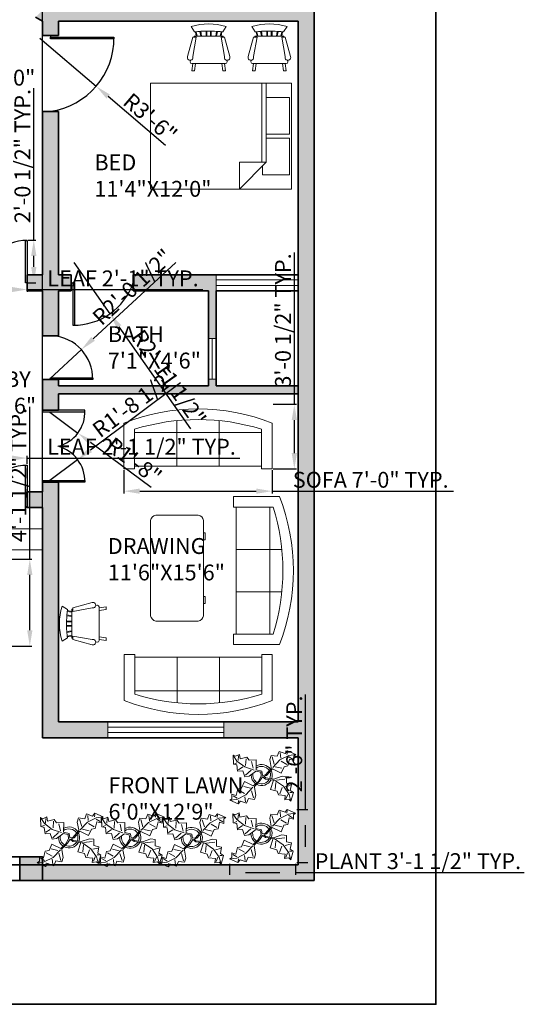
# Model space of a CAD drawing. Units: inches. Extents: x 32476 to 33108, y 58720 to 59630.
# Tile 5 of 6: x 32810 to 33096, y 58720 to 59278. Entities that reach past the tile are written whole.
import ezdxf

# ---------------------------------------------------------------- set-up
doc = ezdxf.new("R2010")
doc.units = ezdxf.units.IN
for name, color, linetype, lineweight in [('A-ANNO-DIMS', 6, 'Continuous', 18), ('A-ANNO-TTLB', 7, 'Continuous', 35), ('A-AREA-IDEN', 32, 'Continuous', 18), ('A-DOOR', 4, 'Continuous', 25), ('A-FLOR-STRS', 7, 'Continuous', 18), ('A-FURN', 8, 'Continuous', 18), ('A-GLAZ', 4, 'Continuous', 18), ('A-SITE-GATE', 7, 'Continuous', 35), ('A-SITE-PATT', 242, 'Continuous', 13), ('A-WALL', 7, 'Continuous', 35), ('A-WALL-PATT', 251, 'Continuous', 13), ('L-PLNT', 3, 'Continuous', 13)]:
    doc.layers.add(name, color=color, linetype=linetype, lineweight=lineweight)
doc.styles.get("Standard").update_dxf_attribs({"font": 'arial.ttf'})
doc.dimstyles.new('ISO-25', dxfattribs={"dimtxt": 9, "dimasz": 9, "dimexe": 1.25, "dimexo": 0.625, "dimtad": 1, "dimdec": 1, "dimrnd": 9, "dimlunit": 3, "dimtxsty": 'Standard', "dimcen": 2.5, "dimadec": 0, "dimazin": 0, "dimtfac": 1, "dimtdec": 1, "dimtmove": 0, "dimatfit": 3, "dimfxl": 1, "dimarcsym": 0})

# ---------------------------------------------------------------- blocks, each defined once
blk = doc.blocks.new('Bed - Queen')
for p, q in [((0, -80.00003), (0, 0)), ((0, 0), (59.99999, 0)), ((59.99999, 0), (59.99999, -80.00003)), ((7.99999, -1.2), (28.79998, -1.2)), ((7.99999, -14.4), (7.99999, -1.2)), ((28.79998, -1.2), (28.79998, -14.4)), ((31.19999, -1.2), (51.99999, -1.2)), ((31.19999, -14.4), (31.19999, -1.2)), ((51.99999, -1.2), (51.99999, -16.4)), ((0, -14.4), (44.8, -14.4)), ((59.99999, -29.6), (44.8, -14.4)), ((44.8, -14.4), (44.8, -29.6)), ((51.99999, -16.4), (46.79936, -16.4)), ((44.8, -16.8), (0, -16.8)), ((44.8, -29.6), (59.99999, -29.6)), ((59.99999, -80.00003), (0, -80.00003))]:
    blk.add_line(p, q)
blk = doc.blocks.new('Chair - Rocking')
for p, q in [((-8, -4.5), (-10, -1.5)), ((-7.5, -4.5), (-7, -7)), ((-6.5, -7), (-7.02225, -4.43)), ((-4.5, -7), (-4.96674, -4.19951)), ((-4, -7), (-4.40532, -4.16272)), ((-1.5, -4.05012), (-1.5, -7)), ((-1, -7), (-1, -4.05012)), ((1, -7), (1, -4.04655)), ((1.5, -4.05012), (1.5, -7)), ((4, -7), (4.40187, -4.18694)), ((4.5, -7), (4.96761, -4.19437)), ((6.5, -7), (7, -4.4057)), ((7.5, -4.5), (7, -7)), ((8, -4.5), (10, -1.5)), ((-9, -7.5), (-12, -18.49999)), ((-7, -7.5), (-9, -7.5)), ((-9, -18.49999), (-7, -7.5)), ((-8.23428, -6.99939), (-8.3093, -7.47958)), ((-8.23041, -7), (8.23915, -7)), ((7, -7.5), (9, -7.5)), ((9, -18.49999), (7, -7.5)), ((8.31071, -7.48854), (8.23449, -7.00073)), ((9, -7.5), (12, -18.49999)), ((-10.36644, -20.64523), (-10.5, -21.49999)), ((10.5, -21.49999), (10.3575, -20.58798)), ((-9, -22.49999), (-9.5, -26.49999)), ((0, -22.49999), (-9.5, -22.49999)), ((-9.5, -26.49999), (-8, -26.49999)), ((-8, -26.49999), (-7.5, -22.49999)), ((0, -22.49999), (9.5, -22.49999)), ((8, -26.49999), (7.5, -22.49999)), ((9.5, -26.49999), (8, -26.49999)), ((9, -22.49999), (9.5, -26.49999))]:
    blk.add_line(p, q)
for centre, radius, start, end in [((0, -34.08333), 34.08333, 72.93847, 107.0615), ((0, -68.25004), 64.25, 93.92211, 97.15267), ((0, -68.25004), 64.25, 82.84733, 93.92211), ((-10.5, -18.99999), 1.58114, 161.5651, 18.43495), ((-9.5, -21.49999), 1, 180, 270), ((10.5, -18.99999), 1.58114, 161.5651, 18.43495), ((9.5, -21.49999), 1, 270, 0)]:
    blk.add_arc(centre, radius, start, end)
blk = doc.blocks.new('Sofa - Roundback 7 ft.')
for p, q in [((-12.00002, -32.4421), (-12.00003, -6.5971)), ((11.99997, -32.4421), (11.99998, -6.5971)), ((-36.000027, -34), (-36.000027, -11.4696)), ((-35.999844, -13.3819), (35.9998, -13.3819)), ((35.99998, -34), (35.99998, -11.4696)), ((-36.000027, -32.4421), (35.99998, -32.4421))]:
    blk.add_line(p, q)
for points in [[(-36.000027, -34), (-42.000027, -34), (-42.000027, -8)], [(41.99998, -8), (41.99998, -34), (35.99998, -34)]]:
    blk.add_lwpolyline(points)
for centre, radius, start, end in [((0, -114.25), 114.25, 68.43141, 111.5686), ((-0.00001, -127.1968), 121.1968, 72.72033, 107.2797)]:
    blk.add_arc(centre, radius, start, end)
blk = doc.blocks.new('Desk - 30 x 60 in.')
for p, q in [((-26.999995, 0), (26.999995, 0)), ((-29.999995, -27), (-29.999995, -3)), ((29.999995, -3), (29.999995, -27)), ((26.999995, -30), (-26.999995, -30)), ((-20.000005, -30), (-20.000005, -31)), ((-20.000005, -31), (-16.000005, -31)), ((-16.000005, -31), (-16.000005, -30)), ((15.999995, -31), (15.999995, -30)), ((19.999995, -31), (15.999995, -31)), ((19.999995, -30), (19.999995, -31))]:
    blk.add_line(p, q)
for centre, start, end in [((-26.499995, -3.5), 98.1301, 171.8699), ((26.499995, -3.5), 8.130102, 81.8699), ((-26.499995, -26.5), 188.1301, 261.8699), ((26.499995, -26.5), 278.1301, 351.8699)]:
    blk.add_arc(centre, 3.535534, start, end)
blk = doc.blocks.new('Plant - Rubber or Philodendron')
for p, q in [((-16.2005, 11.4774), (-13.9899, 8.1064)), ((-16.2005, 11.4774), (-14.8639, 10.7964)), ((-16.0159, 6.3329), (-16.2005, 11.4774)), ((-14.8639, 10.7964), (-12.6195, 11.8975)), ((-12.6195, 11.8975), (-12.1909, 9.4345)), ((4.6914, 8.8812), (5.3859, 11.2828)), ((5.3859, 11.2828), (8.8871, 10.7908)), ((8.8871, 10.7908), (9.9809, 13.4933)), ((9.9809, 13.4933), (13.3837, 12.301)), ((15.3859, 11.3055), (10.3916, 8.7942)), ((10.5828, 12.6946), (10.8893, 9.7953)), ((13.3837, 12.301), (14.68, 13.9039)), ((14.5816, 13.2037), (14.3848, 11.8033)), ((14.68, 13.9039), (19.3848, 11.8146)), ((19.3848, 11.8146), (15.3859, 11.3055)), ((19.3848, 11.8146), (18.1868, 10.9119)), ((-14.0069, 5.8704), (-16.0159, 6.3329)), ((-15.3434, 6.5514), (-13.9984, 6.9884)), ((-13.5868, 2.2894), (-14.0069, 5.8704)), ((-13.9899, 8.1064), (-9.5434, 4.7185)), ((-13.3174, 8.325), (-13.0735, 11.0065)), ((-12.1909, 9.4345), (-8.3829, 10.3)), ((-8.8369, 9.409), (-9.0894, 5.6095)), ((-8.3829, 10.3), (-7.0549, 8.501)), ((-7.0549, 8.501), (-3.0284, 8.6941)), ((-4.8529, 4.012), (-5.7184, 7.82)), ((-3.0284, 8.6941), (-3.0709, 3.1041)), ((4.6914, 8.8812), (5.5014, 4.4831)), ((5.9878, 10.4842), (7.1971, 6.3869)), ((10.3916, 8.7942), (6.2847, 4.4028)), ((14.2977, 6.1031), (10.9934, 7.9956)), ((15.7909, 9.1065), (14.8995, 5.3044)), ((15.2875, 10.6053), (17.5907, 9.2105)), ((18.1925, 8.4119), (15.7909, 9.1065)), ((18.1868, 10.9119), (18.1925, 8.4119)), ((-10.6784, 2.491), (-13.5868, 2.2894)), ((-13.1329, 3.1804), (-10.6614, 4.727)), ((-9.5858, -0.8715), (-10.6784, 2.491)), ((-9.5434, 4.7185), (-4.1917, 2.9888)), ((-9.1318, 0.0195), (-5.9793, 2.9025)), ((-7.1228, -0.443), (-3.5248, 2.2131)), ((-3.5248, 2.2131), (-3.3011, 2.4355)), ((-3.3011, 2.4355), (-0.5306, 1.7947)), ((-3.0709, 3.1041), (0.0797, 2.3163)), ((-0.5306, 1.7947), (-0.2255, -0.5527)), ((-0.5306, 1.7947), (-0.5306, 1.7947)), ((0.0797, 2.3163), (0.4866, -0.031)), ((0.4866, -0.031), (2.1141, 0.2298)), ((2.1141, 0.2298), (5.4346, 3.9146)), ((6.1032, 3.6844), (2.8262, -0.031)), ((5.4346, 3.9146), (5.5014, 4.4831)), ((11.1089, 1.1958), (6.1032, 3.6844)), ((7.7005, 4.8881), (11.5025, 3.9967)), ((12.7005, 4.8994), (11.1089, 1.1958)), ((14.8995, 5.3044), (12.7005, 4.8994)), ((-11.3237, -7.2629), (-9.7321, -3.5593)), ((-9.7321, -3.5593), (-4.7264, -6.0479)), ((-7.1228, -0.443), (-9.5858, -0.8715)), ((-2.019, -3.6148), (-4.7264, -6.0479)), ((-4.0579, -6.2781), (-0.9375, -3.1608)), ((-2.019, -3.6148), (-0.2255, -0.5527)), ((-0.9375, -3.1608), (0.5883, -0.8135)), ((0.5883, -0.8135), (2.2447, -2.0916)), ((2.8262, -0.031), (1.3003, -0.5527)), ((1.3003, -0.5527), (2.4193, -1.4655)), ((2.2447, -2.0916), (6.7108, -2.6626)), ((2.4193, -1.4655), (6.895, -2.1175)), ((4.943, -7.9659), (6.7108, -2.6626)), ((11.6605, -0.5413), (6.895, -2.1175)), ((12.3677, -6.1981), (7.219, -2.6772)), ((8.125, -4.0768), (7.7715, -7.9659)), ((8.3544, -2.7453), (13.1973, -2.1704)), ((11.6605, -0.5413), (14.1354, -0.8948)), ((14.1354, -0.8948), (14.1354, -4.4304)), ((14.1354, -4.4304), (16.9638, -5.1375)), ((16.9638, -5.1375), (16.2567, -8.673)), ((-16.8157, -10.7754), (-14.4141, -11.4699)), ((-16.8101, -13.2754), (-16.8157, -10.7754)), ((-14.4141, -11.4699), (-13.5228, -7.6679)), ((-14.0091, -13.669), (-9.0148, -11.1577)), ((-13.5228, -7.6679), (-11.3237, -7.2629)), ((-12.921, -8.4665), (-9.6166, -10.359)), ((-6.3237, -7.2516), (-10.1257, -6.3602)), ((-9.0148, -11.1577), (-4.9047, -6.8122)), ((-4.611, -12.8477), (-5.8203, -8.7504)), ((-4.1246, -6.8466), (-4.0579, -6.2781)), ((-3.3146, -11.2447), (-4.1246, -6.8466)), ((8.8321, -9.0266), (4.943, -7.9659)), ((9.5392, -11.1479), (8.8321, -9.0266)), ((13.4283, -11.5015), (9.5392, -11.1479)), ((10.2463, -10.4408), (11.6605, -6.9053)), ((15.5496, -10.7943), (12.3677, -6.1981)), ((16.2567, -5.8446), (13.4283, -6.5517)), ((14.8425, -10.7943), (13.7819, -13.2692)), ((16.6103, -14.6834), (15.5496, -10.7943)), ((17.3174, -9.7337), (15.9032, -9.7337)), ((16.2567, -8.673), (18.0245, -9.7337)), ((18.0245, -9.7337), (16.6103, -14.6834)), ((-18.008, -14.1781), (-16.8101, -13.2754)), ((-18.008, -14.1781), (-14.0091, -13.669)), ((-13.3032, -16.2674), (-18.008, -14.1781)), ((-13.9107, -12.9688), (-16.2139, -11.574)), ((-12.0069, -14.6645), (-13.3032, -16.2674)), ((-13.2048, -15.5672), (-13.008, -14.1668)), ((-8.6042, -15.8568), (-12.0069, -14.6645)), ((-9.206, -15.0581), (-9.5126, -12.1588)), ((-7.5103, -13.1543), (-8.6042, -15.8568)), ((-4.0092, -13.6463), (-7.5103, -13.1543)), ((-3.3146, -11.2447), (-4.0092, -13.6463)), ((13.0748, -13.9763), (13.4283, -11.5015)), ((15.5496, -13.6228), (13.0748, -13.9763)), ((16.6103, -14.6834), (15.5496, -13.6228))]:
    blk.add_line(p, q)
for centre, radius, start, end in [((0, 0), 6.1275, 34.37569, 120.1028), ((0.0308, 0.1664), 6, 178.6147, 235.1169), ((0.0308, 0.1664), 5, 168.1647, 238.6725), ((-0.0601, -0.2075), 5.2461, 33.82192, 124.9414), ((-0.2664, 0.1682), 5.2775, 338.4094, 20.03007), ((-0.098, 0.1364), 6.1288, 341.2017, 26.09184), ((-0.0234, 0.3825), 6.1492, 242.5812, 331.2714), ((-0.1102, 0.4886), 5.2883, 247.3711, 327.472)]:
    blk.add_arc(centre, radius, start, end)
blk = doc.blocks.new('DOOR-LOUNGE-PAIRED-LEAF')
for p, q in [((24.2, 0), (24.2, 24)), ((24.2, 24), (25.2, 24)), ((25.2, 24), (25.2, 4.5)), ((25.2, 0), (24.2, 0))]:
    blk.add_line(p, q)
blk.add_arc((24.7, -0.73), 24.73, 88.8415, 177.0325)
blk = doc.blocks.new('DOOR-PORCH-PAIRED-LEAF')
for p, q in [((24.56, 0), (24.56, 24)), ((24.56, 24), (25.56, 24)), ((25.56, 24), (25.56, 9)), ((25.56, 0), (24.56, 0))]:
    blk.add_line(p, q)
blk.add_arc((25.06, -1.08), 25.08, 88.8578, 177.5364)
blk = doc.blocks.new('*D17')
at = {"layer": 'A-ANNO-DIMS', "color": 0, "lineweight": -2, "transparency": 16777216}
for p, q in [((32869.2, 59023.05), (32869.2, 59009.82)), ((32953.2, 59023.05), (32953.2, 59009.82)), ((32878.2, 59011.07), (32944.2, 59011.07)), ((32953.2, 59011.07), (33056, 59011.07))]:
    blk.add_line(p, q, dxfattribs=at)
at = {"layer": 'A-ANNO-DIMS', "color": 0, "transparency": 16777216}
for points in [[(32878.2, 59012.57), (32878.2, 59009.57), (32869.2, 59011.07)], [(32944.2, 59012.57), (32944.2, 59009.57), (32953.2, 59011.07)]]:
    blk.add_solid(points, dxfattribs=at)
at = {"layer": 'Defpoints', "color": 0, "transparency": 16777216}
for p in [(32869.2, 59023.67), (32953.2, 59023.67), (32953.2, 59011.07)]:
    blk.add_point(p, dxfattribs=at)
at = {"layer": 'A-ANNO-DIMS', "color": 0, "transparency": 16777216, "insert": (33009.1, 59016.35), "char_height": 9, "attachment_point": 5}
blk.add_mtext('SOFA 7\'-0" TYP.', dxfattribs=at)
blk = doc.blocks.new('*D18')
at = {"layer": 'A-ANNO-DIMS', "color": 0, "lineweight": -2, "transparency": 16777216}
for p, q in [((32965.8, 59060.34), (32965.8, 59146.41)), ((32953.83, 59060.34), (32967.05, 59060.34)), ((32965.8, 59032.67), (32965.8, 59051.34)), ((32953.83, 59023.67), (32967.05, 59023.67))]:
    blk.add_line(p, q, dxfattribs=at)
at = {"layer": 'A-ANNO-DIMS', "color": 0, "transparency": 16777216}
for points in [[(32964.3, 59051.34), (32967.3, 59051.34), (32965.8, 59060.34)], [(32964.3, 59032.67), (32967.3, 59032.67), (32965.8, 59023.67)]]:
    blk.add_solid(points, dxfattribs=at)
at = {"layer": 'Defpoints', "color": 0, "transparency": 16777216}
for p in [(32953.2, 59060.34), (32965.8, 59060.34), (32953.2, 59023.67)]:
    blk.add_point(p, dxfattribs=at)
at = {"layer": 'A-ANNO-DIMS', "color": 0, "transparency": 16777216, "insert": (32960.52, 59107.88), "char_height": 9, "attachment_point": 5, "rotation": 90}
blk.add_mtext('3\'-0 1/2" TYP.', dxfattribs=at)
blk = doc.blocks.new('*D19')
at = {"layer": 'A-ANNO-DIMS', "color": 0, "lineweight": -2, "transparency": 16777216}
for p, q in [((32929.12, 58799.77), (32929.12, 58793.54)), ((32966.51, 58799.77), (32966.51, 58793.54)), ((32938.12, 58794.79), (32957.51, 58794.79)), ((32966.51, 58794.79), (33096.16, 58794.79))]:
    blk.add_line(p, q, dxfattribs=at)
at = {"layer": 'A-ANNO-DIMS', "color": 0, "transparency": 16777216}
for points in [[(32938.12, 58796.29), (32938.12, 58793.29), (32929.12, 58794.79)], [(32957.51, 58796.29), (32957.51, 58793.29), (32966.51, 58794.79)]]:
    blk.add_solid(points, dxfattribs=at)
at = {"layer": 'Defpoints', "color": 0, "transparency": 16777216}
for p in [(32929.12, 58800.4), (32966.51, 58800.4), (32966.51, 58794.79)]:
    blk.add_point(p, dxfattribs=at)
at = {"layer": 'A-ANNO-DIMS', "color": 0, "transparency": 16777216, "insert": (33035.84, 58800.07), "char_height": 9, "attachment_point": 5}
blk.add_mtext('PLANT 3\'-1 1/2" TYP.', dxfattribs=at)
blk = doc.blocks.new('*D20')
at = {"layer": 'A-ANNO-DIMS', "color": 0, "lineweight": -2, "transparency": 16777216}
for p, q in [((32972.12, 58830.57), (32972.12, 58895.83)), ((32967.14, 58830.57), (32973.37, 58830.57)), ((32972.12, 58809.4), (32972.12, 58821.57)), ((32967.14, 58800.4), (32973.37, 58800.4))]:
    blk.add_line(p, q, dxfattribs=at)
at = {"layer": 'A-ANNO-DIMS', "color": 0, "transparency": 16777216}
for points in [[(32970.62, 58821.57), (32973.62, 58821.57), (32972.12, 58830.57)], [(32970.62, 58809.4), (32973.62, 58809.4), (32972.12, 58800.4)]]:
    blk.add_solid(points, dxfattribs=at)
at = {"layer": 'Defpoints', "color": 0, "transparency": 16777216}
for p in [(32966.51, 58830.57), (32972.12, 58830.57), (32966.51, 58800.4)]:
    blk.add_point(p, dxfattribs=at)
at = {"layer": 'A-ANNO-DIMS', "color": 0, "transparency": 16777216, "insert": (32966.9, 58867.7), "char_height": 9, "attachment_point": 5, "rotation": 90}
blk.add_mtext('2\'-6" TYP.', dxfattribs=at)
blk = doc.blocks.new('*D24')
at = {"layer": 'A-ANNO-DIMS', "color": 0, "lineweight": -2, "transparency": 16777216}
for p, q in [((32815.82, 58972.53), (32815.82, 59058.97)), ((32790.33, 58972.53), (32817.07, 58972.53)), ((32815.82, 58932.18), (32815.82, 58963.53)), ((32790.33, 58923.18), (32817.07, 58923.18))]:
    blk.add_line(p, q, dxfattribs=at)
at = {"layer": 'A-ANNO-DIMS', "color": 0, "transparency": 16777216}
for points in [[(32814.32, 58963.53), (32817.32, 58963.53), (32815.82, 58972.53)], [(32814.32, 58932.18), (32817.32, 58932.18), (32815.82, 58923.18)]]:
    blk.add_solid(points, dxfattribs=at)
at = {"layer": 'Defpoints', "color": 0, "transparency": 16777216}
for p in [(32789.71, 58972.53), (32815.82, 58972.53), (32789.71, 58923.18)]:
    blk.add_point(p, dxfattribs=at)
at = {"layer": 'A-ANNO-DIMS', "color": 0, "transparency": 16777216, "insert": (32810.54, 59020.25), "char_height": 9, "attachment_point": 5, "rotation": 90}
blk.add_mtext('4\'-1 1/2" TYP.', dxfattribs=at)
blk = doc.blocks.new('*D27')
at = {"layer": 'A-ANNO-DIMS', "color": 0, "lineweight": -2, "transparency": 16777216}
for p, q in [((32789.11, 59128.59), (32789.11, 59124.19)), ((32814.31, 59128.59), (32814.31, 59124.19)), ((32798.11, 59125.44), (32805.31, 59125.44)), ((32814.31, 59125.44), (32913.96, 59125.44))]:
    blk.add_line(p, q, dxfattribs=at)
at = {"layer": 'A-ANNO-DIMS', "color": 0, "transparency": 16777216}
for points in [[(32798.11, 59126.94), (32798.11, 59123.94), (32789.11, 59125.44)], [(32805.31, 59126.94), (32805.31, 59123.94), (32814.31, 59125.44)]]:
    blk.add_solid(points, dxfattribs=at)
at = {"layer": 'Defpoints', "color": 0, "transparency": 16777216}
for p in [(32789.11, 59129.22), (32814.31, 59129.22), (32814.31, 59125.44)]:
    blk.add_point(p, dxfattribs=at)
at = {"layer": 'A-ANNO-DIMS', "color": 0, "transparency": 16777216, "insert": (32868.64, 59130.59), "char_height": 9, "attachment_point": 5}
blk.add_mtext('LEAF 2\'-1" TYP.', dxfattribs=at)
blk = doc.blocks.new('*D28')
at = {"layer": 'A-ANNO-DIMS', "color": 0, "lineweight": -2, "transparency": 16777216}
for p, q in [((32818.09, 59153.49), (32818.09, 59239.72)), ((32814.94, 59153.49), (32819.34, 59153.49)), ((32818.09, 59138.22), (32818.09, 59144.49)), ((32814.94, 59129.22), (32819.34, 59129.22))]:
    blk.add_line(p, q, dxfattribs=at)
at = {"layer": 'A-ANNO-DIMS', "color": 0, "transparency": 16777216}
for points in [[(32816.59, 59144.49), (32819.59, 59144.49), (32818.09, 59153.49)], [(32816.59, 59138.22), (32819.59, 59138.22), (32818.09, 59129.22)]]:
    blk.add_solid(points, dxfattribs=at)
at = {"layer": 'Defpoints', "color": 0, "transparency": 16777216}
for p in [(32814.31, 59153.49), (32818.09, 59153.49), (32814.31, 59129.22)]:
    blk.add_point(p, dxfattribs=at)
at = {"layer": 'A-ANNO-DIMS', "color": 0, "transparency": 16777216, "insert": (32812.81, 59201.11), "char_height": 9, "attachment_point": 5, "rotation": 90}
blk.add_mtext('2\'-0 1/2" TYP.', dxfattribs=at)
blk = doc.blocks.new('*D29')
at = {"layer": 'A-ANNO-DIMS', "color": 0, "lineweight": -2, "transparency": 16777216}
for p, q in [((32788.75, 59026.62), (32788.75, 59031.07)), ((32797.75, 59029.82), (32805.31, 59029.82)), ((32814.31, 59026.62), (32814.31, 59031.07)), ((32814.31, 59029.82), (32934.93, 59029.82))]:
    blk.add_line(p, q, dxfattribs=at)
at = {"layer": 'A-ANNO-DIMS', "color": 0, "transparency": 16777216}
for points in [[(32797.75, 59031.32), (32797.75, 59028.32), (32788.75, 59029.82)], [(32805.31, 59031.32), (32805.31, 59028.32), (32814.31, 59029.82)]]:
    blk.add_solid(points, dxfattribs=at)
at = {"layer": 'Defpoints', "color": 0, "transparency": 16777216}
for p in [(32814.31, 59029.82), (32788.75, 59025.99), (32814.31, 59025.99)]:
    blk.add_point(p, dxfattribs=at)
at = {"layer": 'A-ANNO-DIMS', "color": 0, "transparency": 16777216, "insert": (32879.12, 59035.1), "char_height": 9, "attachment_point": 5}
blk.add_mtext('LEAF 2\'-1 1/2" TYP.', dxfattribs=at)
blk = doc.blocks.new('*D43')
at = {"layer": 'A-ANNO-DIMS', "color": 0, "lineweight": -2, "transparency": 16777216}
for p, q in [((32740.73, 58978.34), (32740.73, 59529.47)), ((32823.04, 58978.34), (32823.04, 59529.47)), ((32749.73, 59528.22), (32814.04, 59528.22))]:
    blk.add_line(p, q, dxfattribs=at)
at = {"layer": 'A-ANNO-DIMS', "color": 0, "transparency": 16777216}
for points in [[(32749.73, 59529.72), (32749.73, 59526.72), (32740.73, 59528.22)], [(32814.04, 59529.72), (32814.04, 59526.72), (32823.04, 59528.22)]]:
    blk.add_solid(points, dxfattribs=at)
at = {"layer": 'Defpoints', "color": 0, "transparency": 16777216}
for p in [(32823.04, 59528.22), (32740.73, 58977.72), (32823.04, 58977.72)]:
    blk.add_point(p, dxfattribs=at)
at = {"layer": 'A-ANNO-DIMS', "color": 0, "transparency": 16777216, "insert": (32781.88, 59533.5), "char_height": 9, "attachment_point": 5}
blk.add_mtext('6\'-10 1/2"', dxfattribs=at)
blk = doc.blocks.new('*D55')
at = {"layer": 'A-ANNO-DIMS', "color": 0, "lineweight": -2, "transparency": 16777216}
for p, q in [((32821.58, 59268.02), (32853.45, 59240.73)), ((32892.78, 59207.04), (32860.28, 59234.88))]:
    blk.add_line(p, q, dxfattribs=at)
at = {"layer": 'A-ANNO-DIMS', "color": 0, "transparency": 16777216}
blk.add_solid([(32861.26, 59236.02), (32859.31, 59233.74), (32853.45, 59240.73)], dxfattribs=at)
at = {"layer": 'Defpoints', "color": 0, "transparency": 16777216}
for p in [(32821.58, 59268.02), (32853.45, 59240.73)]:
    blk.add_point(p, dxfattribs=at)
at = {"layer": 'A-ANNO-DIMS', "color": 0, "transparency": 16777216, "insert": (32883.35, 59222), "char_height": 9, "attachment_point": 5, "rotation": 319.4189}
blk.add_mtext('R3\'-6"', dxfattribs=at)
blk = doc.blocks.new('*D57')
at = {"layer": 'A-ANNO-DIMS', "color": 0, "lineweight": -2, "transparency": 16777216}
for p, q in [((32840.79, 59140.8), (32861.25, 59111.69)), ((32907.11, 59046.44), (32866.43, 59104.32))]:
    blk.add_line(p, q, dxfattribs=at)
at = {"layer": 'A-ANNO-DIMS', "color": 0, "transparency": 16777216}
blk.add_solid([(32867.65, 59105.19), (32865.2, 59103.46), (32861.25, 59111.69)], dxfattribs=at)
at = {"layer": 'Defpoints', "color": 0, "transparency": 16777216}
for p in [(32840.79, 59140.8), (32861.25, 59111.69)]:
    blk.add_point(p, dxfattribs=at)
at = {"layer": 'A-ANNO-DIMS', "color": 0, "transparency": 16777216, "insert": (32893.67, 59074.74), "char_height": 9, "attachment_point": 5, "rotation": 305.1019}
blk.add_mtext('R2\'-11 1/2"', dxfattribs=at)
blk = doc.blocks.new('*D58')
at = {"layer": 'A-ANNO-DIMS', "color": 0, "lineweight": -2, "transparency": 16777216}
for p, q in [((32898.53, 59140.71), (32851.69, 59097.45)), ((32827.17, 59074.82), (32845.08, 59091.35))]:
    blk.add_line(p, q, dxfattribs=at)
at = {"layer": 'A-ANNO-DIMS', "color": 0, "transparency": 16777216}
blk.add_solid([(32850.67, 59098.56), (32852.71, 59096.35), (32845.08, 59091.35)], dxfattribs=at)
at = {"layer": 'Defpoints', "color": 0, "transparency": 16777216}
for p in [(32845.08, 59091.35), (32827.17, 59074.82)]:
    blk.add_point(p, dxfattribs=at)
at = {"layer": 'A-ANNO-DIMS', "color": 0, "transparency": 16777216, "insert": (32874.84, 59126.01), "char_height": 9, "attachment_point": 5, "rotation": 42.7159}
blk.add_mtext('R2\'-0 1/2"', dxfattribs=at)
blk = doc.blocks.new('*D59')
at = {"layer": 'A-ANNO-DIMS', "color": 0, "lineweight": -2, "transparency": 16777216}
for p, q in [((32901.28, 59072.48), (32850.16, 59034.37)), ((32826.41, 59016.65), (32842.95, 59028.99))]:
    blk.add_line(p, q, dxfattribs=at)
at = {"layer": 'A-ANNO-DIMS', "color": 0, "transparency": 16777216}
blk.add_solid([(32849.27, 59035.57), (32851.06, 59033.16), (32842.95, 59028.99)], dxfattribs=at)
at = {"layer": 'Defpoints', "color": 0, "transparency": 16777216}
for p in [(32842.95, 59028.99), (32826.41, 59016.65)]:
    blk.add_point(p, dxfattribs=at)
at = {"layer": 'A-ANNO-DIMS', "color": 0, "transparency": 16777216, "insert": (32876.17, 59060.34), "char_height": 9, "attachment_point": 5, "rotation": 36.7094}
blk.add_mtext('R1\'-8 1/2"', dxfattribs=at)
blk = doc.blocks.new('*D60')
at = {"layer": 'A-ANNO-DIMS', "color": 0, "lineweight": -2, "transparency": 16777216}
for p, q in [((32827.12, 59055.94), (32843.11, 59044.03)), ((32884.62, 59013.07), (32850.32, 59038.65))]:
    blk.add_line(p, q, dxfattribs=at)
at = {"layer": 'A-ANNO-DIMS', "color": 0, "transparency": 16777216}
blk.add_solid([(32851.22, 59039.85), (32849.43, 59037.44), (32843.11, 59044.03)], dxfattribs=at)
at = {"layer": 'Defpoints', "color": 0, "transparency": 16777216}
for p in [(32827.12, 59055.94), (32843.11, 59044.03)]:
    blk.add_point(p, dxfattribs=at)
at = {"layer": 'A-ANNO-DIMS', "color": 0, "transparency": 16777216, "insert": (32874.2, 59027.35), "char_height": 9, "attachment_point": 5, "rotation": 323.29}
blk.add_mtext('R1\'-8"', dxfattribs=at)

msp = doc.modelspace()

# ---------------------------------------------------------------- hatches: boundary and pattern name
at = {"layer": 'A-SITE-PATT'}
h = msp.add_hatch(color=256, dxfattribs=at)
h.dxf.hatch_style = 1
h.paths.add_polyline_path([(32605.97, 58803.66), (32593.04, 58803.66), (32593.04, 58790.22), (32605.97, 58790.22)])
h.paths.add_polyline_path([(32766.06, 58799.22), (32753.12, 58799.22), (32753.12, 58790.22), (32766.06, 58790.22)])
h.paths.add_polyline_path([(32766.06, 58803.66), (32753.12, 58803.66), (32753.12, 58799.22), (32766.06, 58799.22)])
h.paths.add_polyline_path([(32823.04, 58799.22), (32810.1, 58799.22), (32810.1, 58790.22), (32823.04, 58790.22)])
h.paths.add_polyline_path([(32823.04, 58803.66), (32810.1, 58803.66), (32810.1, 58799.22), (32823.04, 58799.22)])
at = {"layer": 'A-WALL-PATT'}
h = msp.add_hatch(color=256, dxfattribs=at)
h.dxf.hatch_style = 1
h.paths.add_polyline_path([(32602.04, 59418.72), (32606.39, 59418.72), (32606.39, 59423.22), (32602.04, 59423.22), (32602.04, 59477.22), (32698.04, 59477.22), (32698.04, 59469.73), (32702.54, 59469.73), (32702.54, 59481.72), (32867.54, 59481.72), (32867.54, 59427.72), (32860.2, 59427.72), (32860.2, 59418.72), (32867.54, 59418.72), (32935.14, 59418.72), (32935.14, 59423.22), (32872.04, 59423.22), (32872.04, 59477.22), (32968.04, 59477.22), (32968.04, 59423.22), (32962.36, 59423.22), (32962.36, 59418.72), (32968.04, 59418.72), (32968.04, 59286.72), (32867.54, 59286.72), (32832.04, 59286.72), (32828.7, 59289.44), (32818.99, 59279.82), (32823.04, 59277.72), (32823.04, 59269.52), (32832.04, 59269.52), (32832.04, 59277.72), (32867.54, 59277.72), (32968.04, 59277.72), (32968.04, 58880.22), (32925.88, 58880.22), (32925.88, 58871.22), (32968.04, 58871.22), (32968.04, 58799.22), (32823.04, 58799.22), (32823.04, 58790.22), (32977.04, 58790.22), (32977.04, 59486.22), (32867.54, 59486.22), (32702.54, 59486.22), (32593.04, 59486.22), (32593.04, 58803.66), (32602.04, 58803.66), (32602.04, 59001.72), (32624.39, 59001.72), (32624.39, 59010.72), (32602.04, 59010.72), (32602.04, 59124.72), (32648.65, 59124.72), (32648.65, 59133.72), (32602.04, 59133.72), (32602.04, 59277.72), (32757.41, 59277.72), (32757.41, 59279.22), (32742.07, 59288.84), (32739.6, 59286.72), (32702.54, 59286.72), (32602.04, 59286.72)])
h.paths.add_polyline_path([(32763.92, 59133.72), (32685.69, 59133.72), (32685.69, 59124.72), (32693.04, 59124.72), (32693.04, 59010.72), (32668.87, 59010.72), (32668.87, 59001.72), (32705.76, 59001.72), (32705.76, 59010.72), (32702.04, 59010.72), (32702.04, 59124.72), (32763.92, 59124.72)], flags=17)
h.paths.add_polyline_path([(32832.04, 59226.49), (32823.04, 59226.49), (32823.04, 59133.72), (32814.31, 59133.72), (32814.31, 59124.72), (32823.04, 59124.72), (32823.04, 59099.14), (32832.04, 59099.14), (32832.04, 59124.72), (32839.29, 59124.72), (32839.29, 59133.72), (32832.04, 59133.72)], flags=17)
h.paths.add_polyline_path([(32921.54, 59133.72), (32874.43, 59133.72), (32874.43, 59124.72), (32917.04, 59124.72), (32917.04, 59097.72), (32921.54, 59097.72), (32921.54, 59124.72)], flags=17)
h.paths.add_polyline_path([(32832.04, 59066.22), (32968.04, 59066.22), (32968.04, 59070.72), (32921.54, 59070.72), (32921.54, 59074.56), (32917.04, 59074.56), (32917.04, 59070.72), (32832.04, 59070.72), (32832.04, 59074.32), (32823.04, 59074.32), (32823.04, 59056.98), (32832.04, 59056.98)], flags=17)
h.paths.add_polyline_path([(32738.1, 59010.72), (32721.79, 59010.72), (32721.79, 59001.72), (32738.1, 59001.72)], flags=16)
h.paths.add_polyline_path([(32763.19, 59010.72), (32754.77, 59010.72), (32754.77, 59001.72), (32763.19, 59001.72)], flags=16)
h.paths.add_polyline_path([(32832.04, 59016.15), (32823.04, 59016.15), (32823.04, 59010.72), (32814.31, 59010.72), (32814.31, 59001.72), (32823.04, 59001.72), (32823.04, 58871.22), (32860.05, 58871.22), (32860.05, 58880.22), (32832.04, 58880.22)], flags=17)
h.paths.add_polyline_path([(32702.54, 59448.33), (32698.04, 59448.33), (32698.04, 59423.22), (32631.9, 59423.22), (32631.9, 59418.72), (32702.54, 59418.72), (32706.18, 59418.72), (32706.18, 59427.72), (32702.54, 59427.72)], flags=17)
h.paths.add_polyline_path([(32789.04, 59418.72), (32800.22, 59418.72), (32800.22, 59427.72), (32775.59, 59427.72), (32775.59, 59418.72), (32780.04, 59418.72), (32780.04, 59337.58), (32773.73, 59333.67), (32782.91, 59322.03), (32784.1, 59324.11), (32785.3, 59322.03), (32798.33, 59329.69), (32789.04, 59343.18)], flags=17)

# ---------------------------------------------------------------- linework, layer by layer
at = {"layer": 'A-ANNO-TTLB'}
msp.add_lwpolyline([(32476.39, 59629.64), (33046.1, 59629.64), (33046.1, 58720.03), (32476.39, 58720.03)], close=True, dxfattribs=at)
at = {"layer": 'A-DOOR'}
for p, q in [((32827.54, 59269.52), (32827.54, 59268.52)), ((32827.54, 59268.52), (32863.54, 59268.52)), ((32827.54, 59267.52), (32827.54, 59268.52)), ((32863.54, 59267.52), (32827.54, 59267.52)), ((32863.54, 59268.52), (32863.54, 59267.52)), ((32839.29, 59129.22), (32840.29, 59129.22)), ((32840.29, 59129.22), (32840.29, 59105.22)), ((32841.29, 59129.22), (32840.29, 59129.22)), ((32841.29, 59105.22), (32841.29, 59129.22)), ((32840.29, 59105.22), (32841.29, 59105.22)), ((32827.54, 59074.32), (32827.54, 59075.32)), ((32827.54, 59075.32), (32851.54, 59075.32)), ((32827.54, 59074.32), (32827.54, 59074.32)), ((32851.54, 59074.32), (32832.04, 59074.32)), ((32851.54, 59075.32), (32851.54, 59074.32)), ((32823.04, 59056.98), (32823.04, 59055.98)), ((32823.04, 59055.98), (32847.04, 59055.98)), ((32847.04, 59056.98), (32832.04, 59056.98)), ((32847.04, 59055.98), (32847.04, 59056.98)), ((32823.04, 59016.15), (32823.04, 59017.15)), ((32823.04, 59017.15), (32847.04, 59017.15)), ((32847.04, 59016.15), (32832.04, 59016.15)), ((32847.04, 59017.15), (32847.04, 59016.15))]:
    msp.add_line(p, q, dxfattribs=at)
for centre, radius, start, end in [((32821.58, 59268.02), 41.95, 278.154, 0.6829), ((32840.79, 59140.8), 35.58, 269.1949, 341.009), ((32827.17, 59074.82), 24.37, 358.8244, 86.6068), ((32827.12, 59055.94), 19.94, 283.6091, 2.9731), ((32826.41, 59016.65), 20.63, 358.6115, 74.8062)]:
    msp.add_arc(centre, radius, start, end, dxfattribs=at)
at = {"layer": 'A-FLOR-STRS'}
for p, q in [((32753.73, 58989.72), (32823.04, 58989.72)), ((32740.73, 58977.72), (32823.04, 58977.72))]:
    msp.add_line(p, q, dxfattribs=at)
at = {"layer": 'A-GLAZ'}
for p, q in [((32921.54, 59124.72), (32921.54, 59133.72)), ((32921.54, 59130.93), (32968.04, 59130.93)), ((32921.54, 59127.75), (32968.04, 59127.75)), ((32921.54, 59097.72), (32917.04, 59097.72)), ((32919.29, 59097.72), (32919.29, 59074.56)), ((32917.04, 59074.56), (32921.54, 59074.56)), ((32860.05, 58880.22), (32860.05, 58871.22)), ((32925.88, 58877.22), (32860.05, 58877.22)), ((32925.88, 58880.22), (32925.88, 58871.22)), ((32925.88, 58874.22), (32860.05, 58874.22))]:
    msp.add_line(p, q, dxfattribs=at)
at = {"layer": 'A-SITE-GATE'}
msp.add_line((32766.06, 58803.66), (32810.1, 58803.66), dxfattribs=at)
msp.add_lwpolyline([(32810.1, 58790.22), (32823.04, 58790.22), (32823.04, 58803.66), (32810.1, 58803.66)], close=True, dxfattribs=at)
at = {"layer": 'A-WALL'}
for p, q in [((32977.04, 58790.22), (32977.04, 59486.22)), ((32823.04, 59277.72), (32818.99, 59279.82)), ((32823.04, 59269.52), (32823.04, 59277.72)), ((32832.04, 59277.72), (32867.54, 59277.72)), ((32832.04, 59269.52), (32832.04, 59277.72)), ((32968.04, 59277.72), (32867.54, 59277.72)), ((32968.04, 58880.22), (32968.04, 59277.72)), ((32832.04, 59269.52), (32823.04, 59269.52)), ((32832.04, 59226.49), (32823.04, 59226.49)), ((32823.04, 59133.72), (32823.04, 59226.49)), ((32832.04, 59133.72), (32832.04, 59226.49)), ((32823.04, 59133.72), (32814.31, 59133.72)), ((32814.31, 59124.72), (32814.31, 59133.72)), ((32839.29, 59133.72), (32832.04, 59133.72)), ((32839.29, 59133.72), (32839.29, 59124.72)), ((32968.04, 59133.72), (32874.43, 59133.72)), ((32874.43, 59133.72), (32874.43, 59124.72)), ((32823.04, 59124.72), (32814.31, 59124.72)), ((32823.04, 59099.14), (32823.04, 59124.72)), ((32832.04, 59099.14), (32832.04, 59124.72)), ((32839.29, 59124.72), (32832.04, 59124.72)), ((32917.04, 59124.72), (32874.43, 59124.72)), ((32917.04, 59070.72), (32917.04, 59124.72)), ((32968.04, 59124.72), (32921.54, 59124.72)), ((32921.54, 59070.72), (32921.54, 59124.72)), ((32832.04, 59099.14), (32823.04, 59099.14)), ((32832.04, 59074.32), (32823.04, 59074.32)), ((32823.04, 59056.98), (32823.04, 59074.32)), ((32832.04, 59070.72), (32832.04, 59074.32)), ((32917.04, 59070.72), (32832.04, 59070.72)), ((32968.04, 59066.22), (32832.04, 59066.22)), ((32832.04, 59056.98), (32832.04, 59066.22)), ((32968.04, 59070.72), (32921.54, 59070.72)), ((32832.04, 59056.98), (32823.04, 59056.98)), ((32832.04, 59016.15), (32823.04, 59016.15)), ((32823.04, 59010.72), (32823.04, 59016.15)), ((32832.04, 58880.22), (32832.04, 59016.15)), ((32823.04, 59010.72), (32814.31, 59010.72)), ((32814.31, 59010.72), (32814.31, 59001.72)), ((32823.04, 59001.72), (32814.31, 59001.72)), ((32823.04, 58871.22), (32823.04, 59001.72)), ((32968.04, 58880.22), (32832.04, 58880.22)), ((32968.04, 58871.22), (32823.04, 58871.22)), ((32968.04, 58799.22), (32968.04, 58871.22)), ((32605.97, 58799.22), (32968.04, 58799.22)), ((32593.04, 58790.22), (32977.04, 58790.22))]:
    msp.add_line(p, q, dxfattribs=at)

# ---------------------------------------------------------------- block references
at = {"layer": 'A-DOOR'}
for name, p in [('DOOR-LOUNGE-PAIRED-LEAF', (32789.11, 59129.22)), ('DOOR-PORCH-PAIRED-LEAF', (32788.75, 59001.72))]:
    msp.add_blockref(name, p, dxfattribs=at)
at = {"layer": 'A-FURN'}
for name, p in [('Chair - Rocking', (32917.22, 59276.04)), ('Chair - Rocking', (32951.65, 59276.04)), ('Sofa - Roundback 7 ft.', (32911.2, 59057.67))]:
    msp.add_blockref(name, p, dxfattribs=at)
for name, p, rotation in [('Bed - Queen', (32964.22, 59242.41), 270), ('Sofa - Roundback 7 ft.', (32965.31, 58966.05), 270), ('Desk - 30 x 60 in.', (32884.31, 58967.42), 90), ('Chair - Rocking', (32832.64, 58935.91), 90), ('Sofa - Roundback 7 ft.', (32911.3, 58884.42), 180)]:
    msp.add_blockref(name, p, dxfattribs=dict(at, rotation=rotation))
at = {"layer": 'L-PLNT'}
for p in [(32947.25, 58849.91), (32838.07, 58814.5), (32872.75, 58814.37), (32907.62, 58814.24), (32947.13, 58816.66)]:
    msp.add_blockref('Plant - Rubber or Philodendron', p, dxfattribs=at)

# ---------------------------------------------------------------- texts
at = {"layer": 'A-AREA-IDEN', "char_height": 9, "attachment_point": 1}
for s, width, insert in [('LOUNGE\\P18\'4"X12\'0"', 96.1811, (32752.57, 59265.1)), ('BED \\P11\'4"X12\'0"', 89.8734, (32852.43, 59202.04)), ('BATH\\P7\'1"X4\'6"', 57.3661, (32860.06, 59104.63)), ('ST.LOBBY\\P9\'10"X9\'6"', 92.241, (32759.85, 59079.05)), ('DRAWING\\P11\'6"X15\'6"', 104.5926, (32860.06, 58984.46)), ('FRONT LAWN\\P6\'0"X12\'9"', 106.9702, (32860.44, 58848.76))]:
    msp.add_mtext_dynamic_manual_height_columns(s, width=width, gutter_width=12.5, heights=[0], dxfattribs=dict(at, insert=insert))

# ---------------------------------------------------------------- dimensions: what is measured, and where the dimension line sits
at = {"layer": 'A-ANNO-DIMS'}
dim = msp.add_linear_dim(base=(32823.04, 59528.22), p1=(32740.73, 58977.72), p2=(32823.04, 58977.72), dimstyle='ISO-25', override={"dimdec": 1, "dimlfac": 1, "dimrnd": 0, "dimzin": 1, "dimdsep": 46, "dimlunit": 4, "dimfrac": 2}, dxfattribs=at)
dim.commit()
dim.dimension.update_dxf_attribs({"geometry": '*D43', "text_midpoint": (32781.88, 59533.5)})
for center, mpoint, picture, middle in [((32821.58, 59268.02), (32853.45, 59240.73), '*D55', (32883.35, 59222)), ((32827.17, 59074.82), (32845.08, 59091.35), '*D58', (32874.84, 59126.01)), ((32840.79, 59140.8), (32861.25, 59111.69), '*D57', (32893.67, 59074.74)), ((32826.41, 59016.65), (32842.95, 59028.99), '*D59', (32876.17, 59060.34)), ((32827.12, 59055.94), (32843.11, 59044.03), '*D60', (32874.2, 59027.35))]:
    dim = msp.add_radius_dim(center=center, mpoint=mpoint, dimstyle='ISO-25', override={"dimdec": 1, "dimlfac": 1, "dimrnd": 0, "dimzin": 1, "dimdsep": 46, "dimlunit": 4, "dimfrac": 2}, dxfattribs=at)
    dim.commit()
    dim.dimension.update_dxf_attribs({"geometry": picture, "text_midpoint": middle})
for base, p1, p2, picture, middle in [((32818.09, 59153.49), (32814.31, 59129.22), (32814.31, 59153.49), '*D28', (32812.81, 59201.11)), ((32965.8, 59060.34), (32953.2, 59023.67), (32953.2, 59060.34), '*D18', (32960.52, 59107.88)), ((32815.8223, 58972.5292), (32789.7053, 58923.1843), (32789.7053, 58972.5292), '*D24', (32810.5439, 59020.2507)), ((32972.12, 58830.57), (32966.51, 58800.4), (32966.51, 58830.57), '*D20', (32966.9, 58867.7))]:
    dim = msp.add_linear_dim(base=base, p1=p1, p2=p2, angle=90, text='<> TYP.', dimstyle='ISO-25', override={"dimdec": 1, "dimlfac": 1, "dimrnd": 0, "dimzin": 1, "dimdsep": 46, "dimlunit": 4, "dimfrac": 2}, dxfattribs=at)
    dim.commit()
    dim.dimension.update_dxf_attribs({"geometry": picture, "text_midpoint": middle})
for base, p1, p2, text, picture, middle in [((32814.31, 59125.44), (32789.11, 59129.22), (32814.31, 59129.22), 'LEAF <> TYP.', '*D27', (32868.64, 59130.59)), ((32814.31, 59029.82), (32788.75, 59025.99), (32814.31, 59025.99), 'LEAF <> TYP.', '*D29', (32879.12, 59035.1)), ((32953.2, 59011.07), (32869.2, 59023.67), (32953.2, 59023.67), 'SOFA <> TYP.', '*D17', (33009.1, 59016.35)), ((32966.51, 58794.79), (32929.12, 58800.4), (32966.51, 58800.4), 'PLANT <> TYP.', '*D19', (33035.84, 58800.07))]:
    dim = msp.add_linear_dim(base=base, p1=p1, p2=p2, text=text, dimstyle='ISO-25', override={"dimdec": 1, "dimlfac": 1, "dimrnd": 0, "dimzin": 1, "dimdsep": 46, "dimlunit": 4, "dimfrac": 2}, dxfattribs=at)
    dim.commit()
    dim.dimension.update_dxf_attribs({"geometry": picture, "text_midpoint": middle})

doc.saveas('drawing.dxf')
